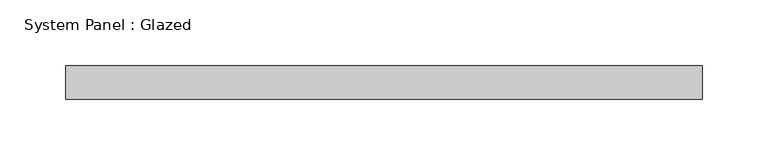
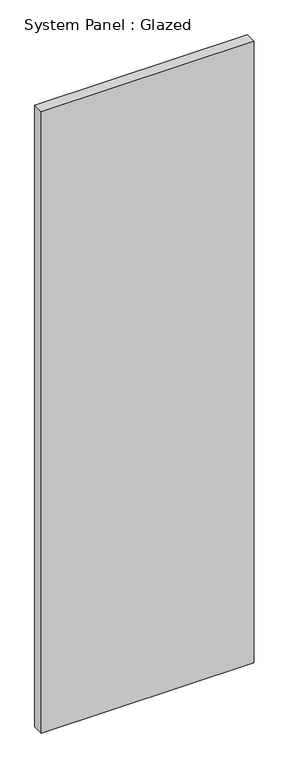
"""IFC4 building model written with IfcOpenShell, lengths in millimetres: plate geometry, System Panel : Glazed."""

from ifc_helpers import new_model, si_unit, origin, origin_with_axes, place, context, project, spatial, polyline, outline, extrude, source, transform, mapped, element, save


def system_panel_glazed_6c57ad35(model_context):
    return source(origin(), model_context, "Body", "SweptSolid", [
        extrude(outline(polyline([(241.3, 19.05), (-241.3, 19.05), (-241.3, 44.45), (241.3, 44.45), (241.3, 19.05)])), origin_with_axes(), (0.0, 0.0, 1.0), 1489.3259354),
    ])


if __name__ == "__main__":
    model = new_model("IFC4")
    model_context = context("Model", 3, world=origin())
    ifc_project = project(units=[si_unit("LENGTHUNIT", "METRE", prefix="MILLI")], contexts=[model_context])
    site = spatial("IfcSite", under=ifc_project)
    building = spatial("IfcBuilding", under=site)
    placement = place(None, origin())
    system_panel_glazed_shape = system_panel_glazed_6c57ad35(model_context)
    element("IfcPlate", 1, ObjectType="System Panel : Glazed", at=placement, inside=building, context=model_context, shape_type="MappedRepresentation", body=[
        mapped(system_panel_glazed_shape, transform((0.0, 0.0, 0.0), x_axis=(1.0, 0.0, 0.0), y_axis=(0.0, 1.0, 0.0), z_axis=(0.0, 0.0, 1.0))),
    ])
    save(model, "model.ifc")

# Revit data of these elements
# Type "System Panel : Glazed"
#   Construction Type Id = "GSP4R"
#   Analytic Construction = "1/8 in Pilkington single glazing"
#   Visual Light Transmittance = 0.9
#   Solar Heat Gain Coefficient = 0.86
#   Heat Transfer Coefficient (U) = 1.18115 BTU/(h·ft²·°F)
#   Define Thermal Properties by = 1
# Element 1 (IfcPlate, "System Panel : Glazed")
#   Materials on its faces: "Glass"
# Materials
#   "Glass": class "Glass", colour RGB 0 128 192, transparency 0.75, Description = "Soda Lime Glass", Cost = 0
